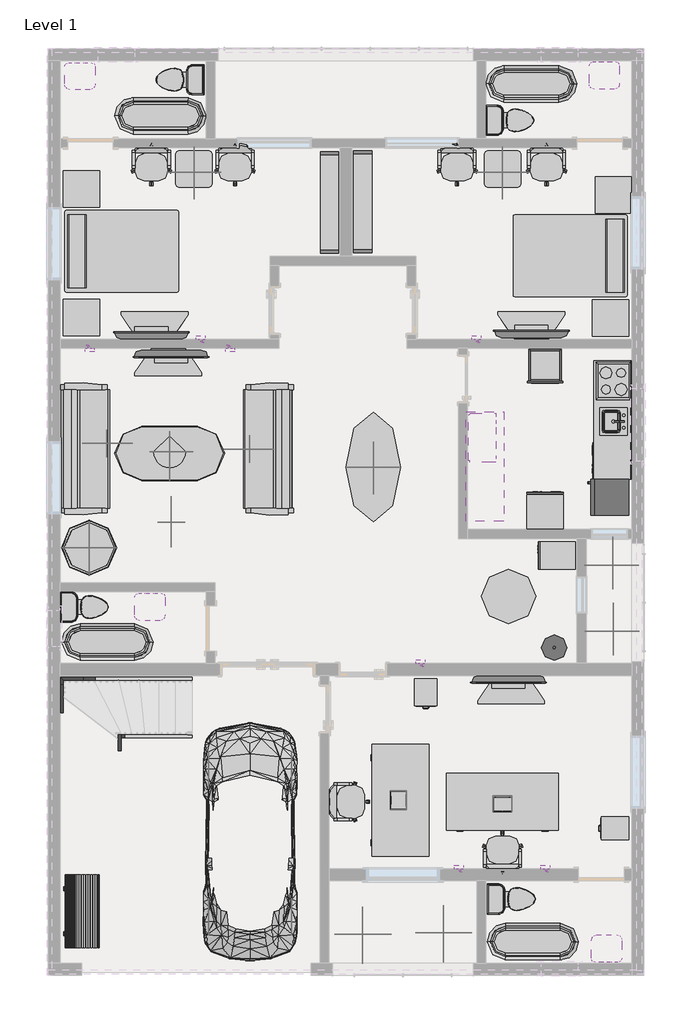
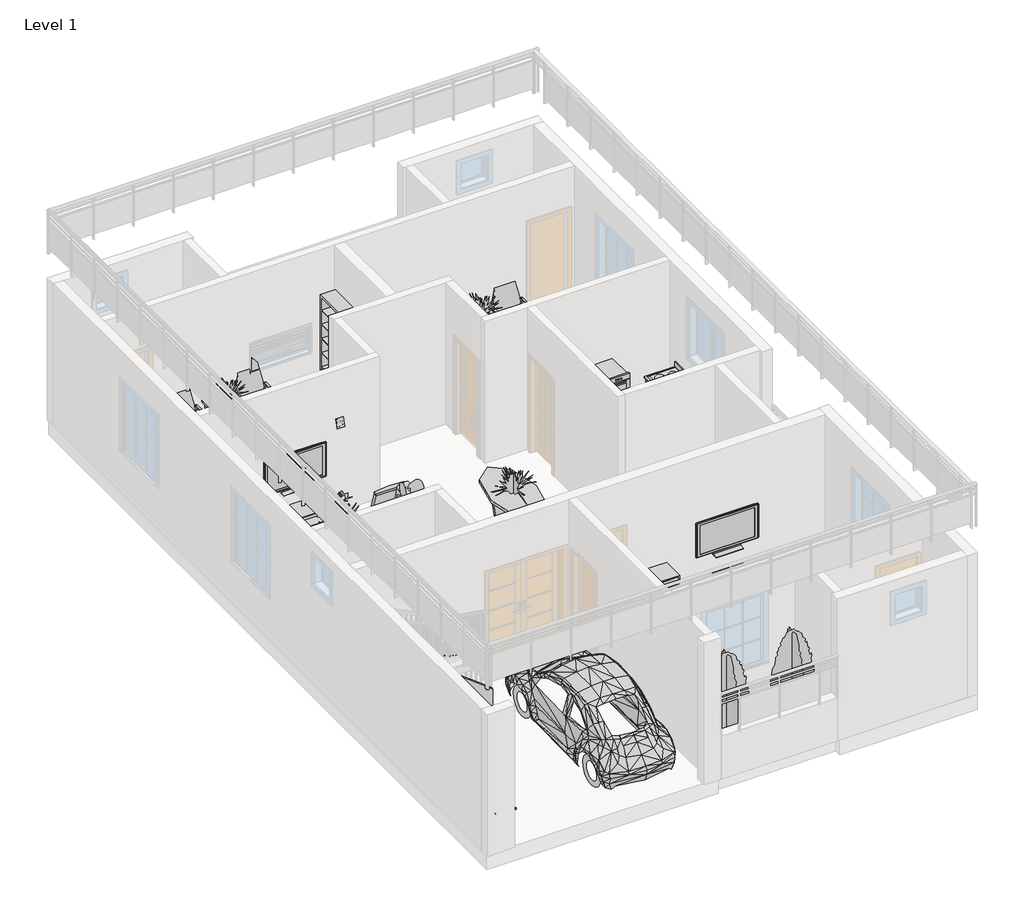
# One storey, part 5 of 5: 36 furniture elements, 22 proxies, 14 flow terminals, 10 geographic elements, 6 members.
# Revit data of these elements (continued)
# Element 29 (IfcFlowTerminal, "Toilet-Domestic-3D : Toilet-Domestic-3D") (continued)
#   Materials on its faces: "Porcelain, Linen", "Laminate, Linen, Matte"
# Element 30 (IfcFlowTerminal, "Toilet-Domestic-3D : Toilet-Domestic-3D")
#   Mark = "5"
#   Phase Created = New Construction
#   Materials on its faces: "Porcelain, Linen", "Laminate, Linen, Matte"
# Element 31 (IfcFlowTerminal, "Toilet-Domestic-3D : Toilet-Domestic-3D")
#   Mark = "8"
#   Phase Created = New Construction
#   Materials on its faces: "Porcelain, Linen", "Laminate, Linen, Matte"
# Element 32 (IfcFlowTerminal, "Toilet-Domestic-3D : Toilet-Domestic-3D")
#   Mark = "11"
#   Phase Created = New Construction
#   Materials on its faces: "Porcelain, Linen", "Laminate, Linen, Matte"
# Element 33 (IfcFlowTerminal, "Tub-Free Standing-3D : 30\" x 60\"")
#   Mark = "2"
#   Phase Created = New Construction
#   Materials on its faces: "Porcelain, Ivory"
# Element 34 (IfcFlowTerminal, "Tub-Free Standing-3D : 30\" x 60\"")
#   Mark = "6"
#   Phase Created = New Construction
#   Materials on its faces: "Porcelain, Ivory"
# Element 35 (IfcFlowTerminal, "Tub-Free Standing-3D : 30\" x 60\"")
#   Mark = "7"
#   Phase Created = New Construction
#   Materials on its faces: "Porcelain, Ivory"
# Element 36 (IfcFlowTerminal, "Tub-Free Standing-3D : 30\" x 60\"")
#   Mark = "12"
#   Phase Created = New Construction
#   Materials on its faces: "Porcelain, Ivory"
# Elements 37, 38 (IfcFurniture, "Bed-Standard.0001 : Double 54\" x 75\"")
#   Phase Created = New Construction
#   Materials on its faces: "Linen, White", "Steel, Chrome Plated"
# Elements 39, 40 (IfcFurniture, "Cabinet-File 3 Drawer.0001 : 15\" x 18\"")
#   Phase Created = New Construction
#   Materials on its faces: "Steel, Chrome Plated", "Steel, Paint Finish, Ivory, Glossy"
# Elements 41, 42, 43, 44, 45, 46 (IfcFurniture, "Chair-Executive : Chair-Executive")
#   Phase Created = New Construction
#   Materials on its faces: "Plastic, Opaque Black", "Textile - Slate Blue"
# Element 47 (IfcFurniture, "Counter Top w Sink Hole : 24\" Depth")
#   Sink Opening Depth = 1' - 2"
#   Sink Location To Wall = 0' - 6"
#   Length = 6' - 6"
#   Sink Location = 3' - 4"
#   Sink Opening Width = 1' - 4"
#   Phase Created = New Construction
#   Materials on its faces: "Counter Top"
# Element 48 (IfcFurniture, "Counter Top w Sink Hole : 24\" Depth")
#   Sink Opening Width = 2' - 3"
#   Sink Opening Depth = 1' - 3"
#   Sink Location To Wall = 0' - 6"
#   Sink Location = 2' - 0"
#   Length = 6' - 0"
#   Phase Created = New Construction
#   Materials on its faces: "Counter Top"
# Elements 49, 50 (IfcFurniture, "Desk : 72\" x 36\"")
#   Phase Created = New Construction
#   Materials on its faces: "Steel, Chrome Plated", "Laminate, Ivory, Matte", "Cherry"
# Elements 51, 52 (IfcFurniture, "Shelving : 96\" x 12\" x 84\"")
#   Phase Created = New Construction
#   Materials on its faces: "Laminate, Ivory, Matte"
# Elements 53, 54 (IfcFurniture, "Sofa-Pensi : 84\"")
#   Phase Created = New Construction
#   Materials on its faces: "Cherry", "Linen, Beige", "Steel, Chrome Plated"
# Elements 55, 56, 57, 58 (IfcFurniture, "TV - Flat Screen : 50\"")
#   Stand = yes
#   Phase Created = New Construction
#   Materials on its faces: "TV - Black", "TV - Glass", "TV - Screen"
# Elements 59, 60, 61, 62 (IfcFurniture, "TV Stand : TV Stand")
#   Phase Created = New Construction
#   Materials on its faces: "Melamine - Gray", "Glass - Shelves"
# Element 63 (IfcFurniture, "Table-Dining Oval : 36\" x 72\"")
#   Phase Created = New Construction
#   Materials on its faces: "Steel, Chrome Plated", "Glass - Clear, Grey"
# Element 64 (IfcFurniture, "Table-Dining Round w Chairs : 36\" Diameter")
#   Phase Created = New Construction
#   Materials on its faces: "Pine", "Laminate, Linen, Matte"
# Element 65 (IfcFurniture, "Table-Ellipse : 72\" x 36\"")
#   Phase Created = New Construction
#   Materials on its faces: "Birch", "Laminate - Black"
# Elements 66, 67 (IfcFurniture, "Table-End : 24\" x 24\"")
#   Phase Created = New Construction
#   Materials on its faces: "Laminate, Ivory, Matte", "Birch"
# Elements 68, 69, 70, 71 (IfcFurniture, "Table-Night Stand : 24\" x 24\" x 30\"")
#   Phase Created = New Construction
#   Materials on its faces: "Birch", "Laminate, Ivory, Matte"
# Element 72 (IfcFurniture, "Table-Round : 36\" Diameter")
#   Phase Created = New Construction
#   Materials on its faces: "Steel, Chrome Plated", "Birch"
# Element 73 (IfcGeographicElement, "Park Bench : 72\"")
#   Phase Created = New Construction
#   Materials on its faces: "Wood - Teak", "Steel, Paint Finish, Dark Gray, Matte"
# Element 74 (IfcGeographicElement, "RPC Plant - Tropical")
#   Phase Created = New Construction
# Elements 75, 76, 77, 78 (IfcGeographicElement, "RPC Plant - Tropical : Agave - 1.5'")
#   Phase Created = New Construction
# Elements 79, 80 (IfcGeographicElement, "RPC Plant - Tropical : Jungle Flame - 3'")
#   Phase Created = New Construction
# Elements 81, 82 (IfcGeographicElement, "RPC Tree - Conifer : Chinese Juniper - 7'")
#   Phase Created = New Construction
# Elements 83, 84, 85, 86, 87, 88 (IfcMember, "Stringer - 2\" Width")
#   Phase Created = New Construction
# Materials
#   "Plastic, Opaque Black": class "Plastic", colour RGB 0 0 0, transparency 0, Description = "Plastic, generic, opaque black", Cost = 0
#   "Steel, Paint Finish, Ivory, Matte": class "Metal", colour RGB 247 247 239, transparency 0, Description = "Steel, paint finish, ivory, matte", Cost = 0
#   "Steel, Chrome Plated": class "Metal", colour RGB 17 17 17, transparency 0, Description = "Chromiuim plated steel", Cost = 0
#   "Steel, Polished": class "Metal", colour RGB 57 57 57, transparency 0, Description = "Polished steel", Cost = 0
#   "Steel, Paint Finish, Ivory, Glossy": class "Metal", colour RGB 247 247 239, transparency 0, Description = "Steel, paint finish, ivory, glossy", Cost = 0
#   "Cabinets": colour RGB 249 249 249, transparency 0
#   "Cabinets - Handles": class "Metal", colour RGB 57 57 57, transparency 0
#   "Laminate, Ivory, Matte": class "Plastic", colour RGB 247 247 239, transparency 0, Description = "Plastic Laminate - Ivory, Matte", Cost = 0
#   "Metal - Stainless Steel, Polished": class "Metal", colour RGB 216 216 216, transparency 0
#   "Porcelain, Linen": class "Ceramic", colour RGB 249 239 230, transparency 0, Description = "Porcelain, linen", Cost = 0
#   "Laminate, Linen, Matte": class "Plastic", colour RGB 249 239 230, transparency 0, Description = "Plastic Laminate - Linen, Matte", Cost = 0
#   "Porcelain, Ivory": class "Ceramic", colour RGB 247 247 239, transparency 0, Description = "Porcelain, ivory", Cost = 0
#   "Textile - Slate Blue": class "Fabric", colour RGB 98 102 118, transparency 0
#   "Cherry": class "Wood", colour RGB 226 177 128, transparency 0, Description = "Prunus Serotina", Cost = 0
#   "Linen, Beige": class "Textile", colour RGB 249 239 230, transparency 0, Description = "Linen, beige", Cost = 0
#   "Melamine - Gray": class "Wood", colour RGB 49 49 49, transparency 0
#   "Glass - Clear, Grey": class "Glass", colour RGB 252 255 255, transparency 0.64
#   "Pine": class "Wood", colour RGB 223 192 134, transparency 0, Description = "Pinus Echinata", Cost = 0
#   "Birch": class "Wood", colour RGB 224 178 126, transparency 0, Description = "Betula Alleghaniensis", Cost = 0
#   "Laminate - Black": colour RGB 0 0 0, transparency 0
#   "Wood - Teak": class "Wood", colour RGB 120 73 19, transparency 0
#   "Steel, Paint Finish, Dark Gray, Matte": class "Metal", colour RGB 98 98 98, transparency 0, Description = "Steel, paint finish, dark gray, matte", Cost = 0
#   "Default Mass Zone": class "Generic", colour RGB 0 255 0, transparency 0.5, Cost = 0
#   "Glass": class "Glass", colour RGB 0 128 192, transparency 0.75, Description = "Soda Lime Glass", Cost = 0
#   "Steel": class "Metal", colour RGB 247 247 247, transparency 0, Description = "Steel, mill finish", Cost = 0
#   "Linen, White": class "Textile", colour RGB 247 247 239, transparency 0, Description = "Linen, white", Cost = 0
#   "Counter Top": class "Wood", colour RGB 226 177 128, transparency 0
#   "TV - Black": colour RGB 49 49 49, transparency 0
#   "TV - Glass": colour RGB 157 157 157, transparency 0.9
#   "TV - Screen": colour RGB 0 0 0, transparency 0
#   "Glass - Shelves": class "Glass", colour RGB 167 167 167, transparency 0.9
